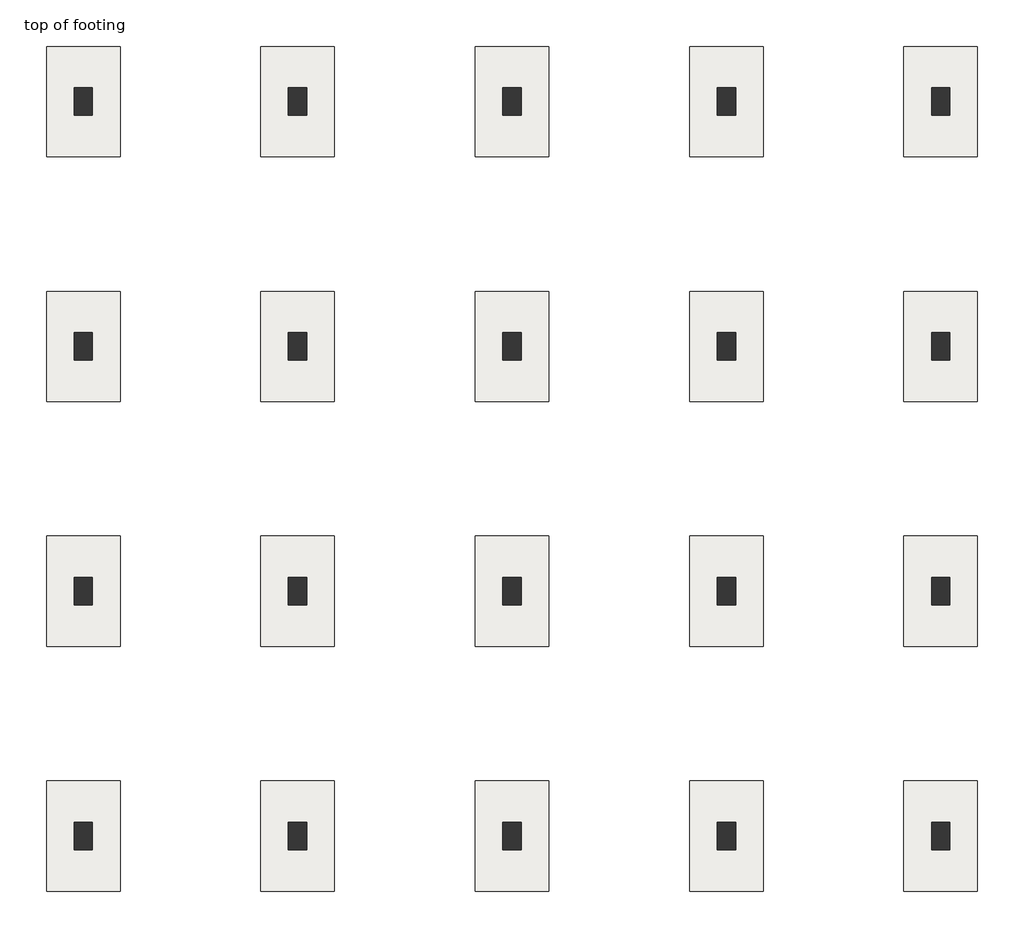
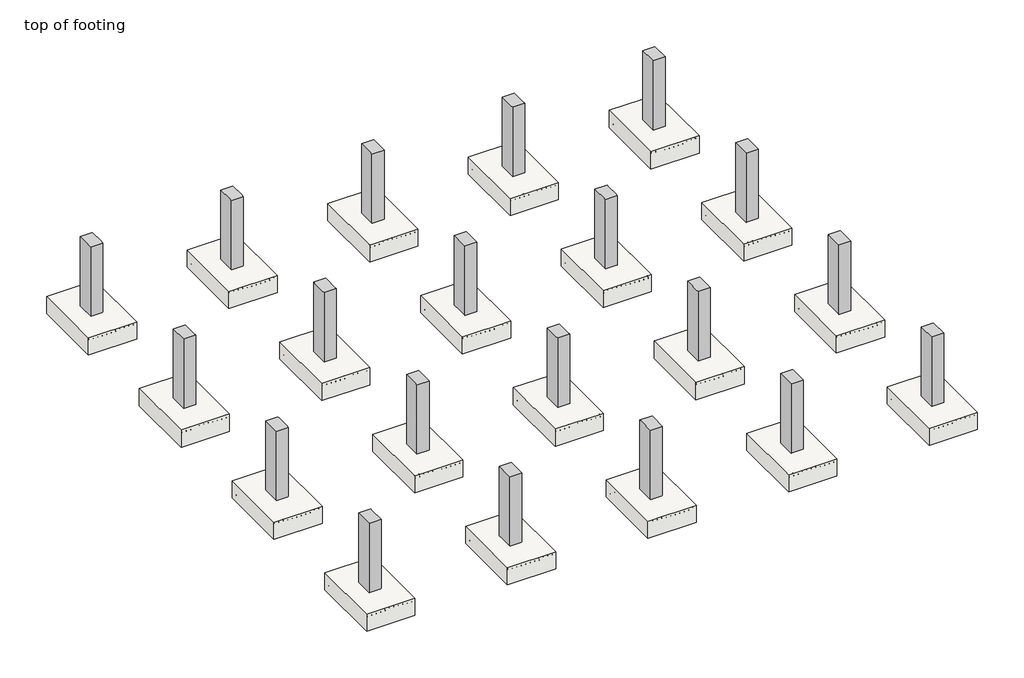
# One storey, part 1 of 8: 20 columns, 20 slabs.
"""IFC4 building model written with IfcOpenShell, lengths in millimetres."""

from ifc_helpers import new_model, si_unit, origin, place, context, project, spatial, faceted_brep, transform, mapped, element, save
from components import m_footing_rectangular_1800_x_1200_x_450mm_16ba7ea5

model = new_model("IFC4")

# Units and contexts
model_context = context("Model", 3, world=origin())
ifc_project = project(units=[si_unit("LENGTHUNIT", "METRE", prefix="MILLI")], contexts=[model_context])

# Site, building, storey
site = spatial("IfcSite", under=ifc_project)
building = spatial("IfcBuilding", under=site)
storey = spatial("IfcBuildingStorey", under=building, Name="top of footing", Elevation=-1828.8)

# Columns
placement = place(None, origin())
element("IfcColumn", 1, ObjectType="M_Concrete-Rectangular-Column : 300 x 450mm", at=placement, inside=storey, context=model_context, shape_type="Brep", body=[
    faceted_brep([(-11089.0800189, 17761.4575251, -1828.8), (-11089.0800189, 17311.4575251, -1828.8), (-11389.0800189, 17311.4575251, -1828.8), (-11389.0800189, 17761.4575251, -1828.8), (-11089.0800189, 17761.4575251, 0.0), (-11089.0800189, 17386.4575251, 0.0), (-11089.0800189, 17311.4575251, 0.0), (-11389.0800189, 17311.4575251, 0.0), (-11389.0800189, 17761.4575251, 0.0)], [[[0, 1, 2, 3]], [[4, 5, 6, 1, 0]], [[6, 7, 2, 1]], [[7, 8, 3, 2]], [[8, 4, 0, 3]], [[4, 8, 7, 6, 5]]]),
])
element("IfcColumn", 2, ObjectType="M_Concrete-Rectangular-Column : 300 x 450mm", at=placement, inside=storey, context=model_context, shape_type="Brep", body=[
    faceted_brep([(-11089.0800189, 13761.4575251, -1828.8), (-11089.0800189, 13311.4575251, -1828.8), (-11389.0800189, 13311.4575251, -1828.8), (-11389.0800189, 13761.4575251, -1828.8), (-11089.0800189, 13761.4575251, 0.0), (-11089.0800189, 13686.4575251, 0.0), (-11089.0800189, 13386.4575251, 0.0), (-11089.0800189, 13311.4575251, 0.0), (-11389.0800189, 13311.4575251, 0.0), (-11389.0800189, 13761.4575251, 0.0)], [[[0, 1, 2, 3]], [[4, 5, 6, 7, 1, 0]], [[7, 8, 2, 1]], [[8, 9, 3, 2]], [[9, 4, 0, 3]], [[4, 9, 8, 7, 6, 5]]]),
])
element("IfcColumn", 3, ObjectType="M_Concrete-Rectangular-Column : 300 x 450mm", at=placement, inside=storey, context=model_context, shape_type="Brep", body=[
    faceted_brep([(-11089.0800189, 9761.4575251, -1828.8), (-11089.0800189, 9311.4575251, -1828.8), (-11389.0800189, 9311.4575251, -1828.8), (-11389.0800189, 9761.4575251, -1828.8), (-11089.0800189, 9761.4575251, 0.0), (-11089.0800189, 9686.4575251, 0.0), (-11089.0800189, 9386.4575251, 0.0), (-11089.0800189, 9311.4575251, 0.0), (-11389.0800189, 9311.4575251, 0.0), (-11389.0800189, 9761.4575251, 0.0)], [[[0, 1, 2, 3]], [[4, 5, 6, 7, 1, 0]], [[7, 8, 2, 1]], [[8, 9, 3, 2]], [[9, 4, 0, 3]], [[4, 9, 8, 7, 6, 5]]]),
])
element("IfcColumn", 4, ObjectType="M_Concrete-Rectangular-Column : 300 x 450mm", at=placement, inside=storey, context=model_context, shape_type="Brep", body=[
    faceted_brep([(-11089.0800189, 5761.4575251, -1828.8), (-11089.0800189, 5311.4575251, -1828.8), (-11389.0800189, 5311.4575251, -1828.8), (-11389.0800189, 5761.4575251, -1828.8), (-11089.0800189, 5761.4575251, 0.0), (-11089.0800189, 5686.4575251, 0.0), (-11089.0800189, 5311.4575251, 0.0), (-11389.0800189, 5311.4575251, 0.0), (-11389.0800189, 5761.4575251, 0.0)], [[[0, 1, 2, 3]], [[4, 5, 6, 1, 0]], [[6, 7, 2, 1]], [[7, 8, 3, 2]], [[8, 4, 0, 3]], [[4, 8, 7, 6, 5]]]),
])
element("IfcColumn", 5, ObjectType="M_Concrete-Rectangular-Column : 300 x 450mm", at=placement, inside=storey, context=model_context, shape_type="Brep", body=[
    faceted_brep([(-7589.0800189, 17761.4575251, -1828.8), (-7589.0800189, 17311.4575251, -1828.8), (-7889.0800189, 17311.4575251, -1828.8), (-7889.0800189, 17761.4575251, -1828.8), (-7589.0800189, 17761.4575251, 0.0), (-7589.0800189, 17386.4575251, 0.0), (-7589.0800189, 17311.4575251, 0.0), (-7889.0800189, 17311.4575251, 0.0), (-7889.0800189, 17386.4575251, 0.0), (-7889.0800189, 17761.4575251, 0.0)], [[[0, 1, 2, 3]], [[4, 5, 6, 1, 0]], [[6, 7, 2, 1]], [[7, 8, 9, 3, 2]], [[9, 4, 0, 3]], [[4, 9, 8, 7, 6, 5]]]),
])
element("IfcColumn", 6, ObjectType="M_Concrete-Rectangular-Column : 300 x 450mm", at=placement, inside=storey, context=model_context, shape_type="Brep", body=[
    faceted_brep([(-7589.0800189, 13761.4575251, -1828.8), (-7589.0800189, 13311.4575251, -1828.8), (-7889.0800189, 13311.4575251, -1828.8), (-7889.0800189, 13761.4575251, -1828.8), (-7589.0800189, 13761.4575251, 0.0), (-7589.0800189, 13686.4575251, 0.0), (-7589.0800189, 13386.4575251, 0.0), (-7589.0800189, 13311.4575251, 0.0), (-7889.0800189, 13311.4575251, 0.0), (-7889.0800189, 13386.4575251, 0.0), (-7889.0800189, 13686.4575251, 0.0), (-7889.0800189, 13761.4575251, 0.0)], [[[0, 1, 2, 3]], [[4, 5, 6, 7, 1, 0]], [[7, 8, 2, 1]], [[8, 9, 10, 11, 3, 2]], [[11, 4, 0, 3]], [[4, 11, 10, 9, 8, 7, 6, 5]]]),
])
element("IfcColumn", 7, ObjectType="M_Concrete-Rectangular-Column : 300 x 450mm", at=placement, inside=storey, context=model_context, shape_type="Brep", body=[
    faceted_brep([(-7589.0800189, 9761.4575251, -1828.8), (-7589.0800189, 9311.4575251, -1828.8), (-7889.0800189, 9311.4575251, -1828.8), (-7889.0800189, 9761.4575251, -1828.8), (-7589.0800189, 9761.4575251, 0.0), (-7589.0800189, 9686.4575251, 0.0), (-7589.0800189, 9386.4575251, 0.0), (-7589.0800189, 9311.4575251, 0.0), (-7889.0800189, 9311.4575251, 0.0), (-7889.0800189, 9386.4575251, 0.0), (-7889.0800189, 9686.4575251, 0.0), (-7889.0800189, 9761.4575251, 0.0)], [[[0, 1, 2, 3]], [[4, 5, 6, 7, 1, 0]], [[7, 8, 2, 1]], [[8, 9, 10, 11, 3, 2]], [[11, 4, 0, 3]], [[4, 11, 10, 9, 8, 7, 6, 5]]]),
])
element("IfcColumn", 8, ObjectType="M_Concrete-Rectangular-Column : 300 x 450mm", at=placement, inside=storey, context=model_context, shape_type="Brep", body=[
    faceted_brep([(-7589.0800189, 5761.4575251, -1828.8), (-7589.0800189, 5311.4575251, -1828.8), (-7889.0800189, 5311.4575251, -1828.8), (-7889.0800189, 5761.4575251, -1828.8), (-7589.0800189, 5761.4575251, 0.0), (-7589.0800189, 5686.4575251, 0.0), (-7589.0800189, 5311.4575251, 0.0), (-7889.0800189, 5311.4575251, 0.0), (-7889.0800189, 5686.4575251, 0.0), (-7889.0800189, 5761.4575251, 0.0)], [[[0, 1, 2, 3]], [[4, 5, 6, 1, 0]], [[6, 7, 2, 1]], [[7, 8, 9, 3, 2]], [[9, 4, 0, 3]], [[4, 9, 8, 7, 6, 5]]]),
])
element("IfcColumn", 9, ObjectType="M_Concrete-Rectangular-Column : 300 x 450mm", at=placement, inside=storey, context=model_context, shape_type="Brep", body=[
    faceted_brep([(-4089.0800189, 17761.4575251, -1828.8), (-4089.0800189, 17311.4575251, -1828.8), (-4389.0800189, 17311.4575251, -1828.8), (-4389.0800189, 17761.4575251, -1828.8), (-4089.0800189, 17761.4575251, 0.0), (-4089.0800189, 17386.4575251, 0.0), (-4089.0800189, 17311.4575251, 0.0), (-4389.0800189, 17311.4575251, 0.0), (-4389.0800189, 17386.4575251, 0.0), (-4389.0800189, 17761.4575251, 0.0)], [[[0, 1, 2, 3]], [[4, 5, 6, 1, 0]], [[6, 7, 2, 1]], [[7, 8, 9, 3, 2]], [[9, 4, 0, 3]], [[4, 9, 8, 7, 6, 5]]]),
])
element("IfcColumn", 10, ObjectType="M_Concrete-Rectangular-Column : 300 x 450mm", at=placement, inside=storey, context=model_context, shape_type="Brep", body=[
    faceted_brep([(-4089.0800189, 13761.4575251, -1828.8), (-4089.0800189, 13311.4575251, -1828.8), (-4389.0800189, 13311.4575251, -1828.8), (-4389.0800189, 13761.4575251, -1828.8), (-4089.0800189, 13761.4575251, 0.0), (-4089.0800189, 13686.4575251, 0.0), (-4089.0800189, 13386.4575251, 0.0), (-4089.0800189, 13311.4575251, 0.0), (-4389.0800189, 13311.4575251, 0.0), (-4389.0800189, 13386.4575251, 0.0), (-4389.0800189, 13686.4575251, 0.0), (-4389.0800189, 13761.4575251, 0.0)], [[[0, 1, 2, 3]], [[4, 5, 6, 7, 1, 0]], [[7, 8, 2, 1]], [[8, 9, 10, 11, 3, 2]], [[11, 4, 0, 3]], [[4, 11, 10, 9, 8, 7, 6, 5]]]),
])
element("IfcColumn", 11, ObjectType="M_Concrete-Rectangular-Column : 300 x 450mm", at=placement, inside=storey, context=model_context, shape_type="Brep", body=[
    faceted_brep([(-4089.0800189, 9761.4575251, -1828.8), (-4089.0800189, 9311.4575251, -1828.8), (-4389.0800189, 9311.4575251, -1828.8), (-4389.0800189, 9761.4575251, -1828.8), (-4089.0800189, 9761.4575251, 0.0), (-4089.0800189, 9686.4575251, 0.0), (-4089.0800189, 9386.4575251, 0.0), (-4089.0800189, 9311.4575251, 0.0), (-4389.0800189, 9311.4575251, 0.0), (-4389.0800189, 9386.4575251, 0.0), (-4389.0800189, 9686.4575251, 0.0), (-4389.0800189, 9761.4575251, 0.0)], [[[0, 1, 2, 3]], [[4, 5, 6, 7, 1, 0]], [[7, 8, 2, 1]], [[8, 9, 10, 11, 3, 2]], [[11, 4, 0, 3]], [[4, 11, 10, 9, 8, 7, 6, 5]]]),
])
element("IfcColumn", 12, ObjectType="M_Concrete-Rectangular-Column : 300 x 450mm", at=placement, inside=storey, context=model_context, shape_type="Brep", body=[
    faceted_brep([(-4089.0800189, 5761.4575251, -1828.8), (-4089.0800189, 5311.4575251, -1828.8), (-4389.0800189, 5311.4575251, -1828.8), (-4389.0800189, 5761.4575251, -1828.8), (-4089.0800189, 5761.4575251, 0.0), (-4089.0800189, 5686.4575251, 0.0), (-4089.0800189, 5311.4575251, 0.0), (-4389.0800189, 5311.4575251, 0.0), (-4389.0800189, 5686.4575251, 0.0), (-4389.0800189, 5761.4575251, 0.0)], [[[0, 1, 2, 3]], [[4, 5, 6, 1, 0]], [[6, 7, 2, 1]], [[7, 8, 9, 3, 2]], [[9, 4, 0, 3]], [[4, 9, 8, 7, 6, 5]]]),
])
element("IfcColumn", 13, ObjectType="M_Concrete-Rectangular-Column : 300 x 450mm", at=placement, inside=storey, context=model_context, shape_type="Brep", body=[
    faceted_brep([(-589.0800189, 17761.4575251, -1828.8), (-589.0800189, 17311.4575251, -1828.8), (-889.0800189, 17311.4575251, -1828.8), (-889.0800189, 17761.4575251, -1828.8), (-589.0800189, 17761.4575251, 0.0), (-589.0800189, 17386.4575251, 0.0), (-589.0800189, 17311.4575251, 0.0), (-889.0800189, 17311.4575251, 0.0), (-889.0800189, 17386.4575251, 0.0), (-889.0800189, 17761.4575251, 0.0)], [[[0, 1, 2, 3]], [[4, 5, 6, 1, 0]], [[6, 7, 2, 1]], [[7, 8, 9, 3, 2]], [[9, 4, 0, 3]], [[4, 9, 8, 7, 6, 5]]]),
])
element("IfcColumn", 14, ObjectType="M_Concrete-Rectangular-Column : 300 x 450mm", at=placement, inside=storey, context=model_context, shape_type="Brep", body=[
    faceted_brep([(-589.0800189, 13761.4575251, -1828.8), (-589.0800189, 13311.4575251, -1828.8), (-889.0800189, 13311.4575251, -1828.8), (-889.0800189, 13761.4575251, -1828.8), (-589.0800189, 13761.4575251, 0.0), (-589.0800189, 13686.4575251, 0.0), (-589.0800189, 13386.4575251, 0.0), (-589.0800189, 13311.4575251, 0.0), (-889.0800189, 13311.4575251, 0.0), (-889.0800189, 13386.4575251, 0.0), (-889.0800189, 13686.4575251, 0.0), (-889.0800189, 13761.4575251, 0.0)], [[[0, 1, 2, 3]], [[4, 5, 6, 7, 1, 0]], [[7, 8, 2, 1]], [[8, 9, 10, 11, 3, 2]], [[11, 4, 0, 3]], [[4, 11, 10, 9, 8, 7, 6, 5]]]),
])
element("IfcColumn", 15, ObjectType="M_Concrete-Rectangular-Column : 300 x 450mm", at=placement, inside=storey, context=model_context, shape_type="Brep", body=[
    faceted_brep([(-589.0800189, 9761.4575251, -1828.8), (-589.0800189, 9311.4575251, -1828.8), (-889.0800189, 9311.4575251, -1828.8), (-889.0800189, 9761.4575251, -1828.8), (-589.0800189, 9761.4575251, 0.0), (-589.0800189, 9686.4575251, 0.0), (-589.0800189, 9386.4575251, 0.0), (-589.0800189, 9311.4575251, 0.0), (-889.0800189, 9311.4575251, 0.0), (-889.0800189, 9386.4575251, 0.0), (-889.0800189, 9686.4575251, 0.0), (-889.0800189, 9761.4575251, 0.0)], [[[0, 1, 2, 3]], [[4, 5, 6, 7, 1, 0]], [[7, 8, 2, 1]], [[8, 9, 10, 11, 3, 2]], [[11, 4, 0, 3]], [[4, 11, 10, 9, 8, 7, 6, 5]]]),
])
element("IfcColumn", 16, ObjectType="M_Concrete-Rectangular-Column : 300 x 450mm", at=placement, inside=storey, context=model_context, shape_type="Brep", body=[
    faceted_brep([(-589.0800189, 5761.4575251, -1828.8), (-589.0800189, 5311.4575251, -1828.8), (-889.0800189, 5311.4575251, -1828.8), (-889.0800189, 5761.4575251, -1828.8), (-589.0800189, 5761.4575251, 0.0), (-589.0800189, 5686.4575251, 0.0), (-589.0800189, 5311.4575251, 0.0), (-889.0800189, 5311.4575251, 0.0), (-889.0800189, 5686.4575251, 0.0), (-889.0800189, 5761.4575251, 0.0)], [[[0, 1, 2, 3]], [[4, 5, 6, 1, 0]], [[6, 7, 2, 1]], [[7, 8, 9, 3, 2]], [[9, 4, 0, 3]], [[4, 9, 8, 7, 6, 5]]]),
])
element("IfcColumn", 17, ObjectType="M_Concrete-Rectangular-Column : 300 x 450mm", at=placement, inside=storey, context=model_context, shape_type="Brep", body=[
    faceted_brep([(2910.9199811, 17761.4575251, -1828.8), (2910.9199811, 17311.4575251, -1828.8), (2610.9199811, 17311.4575251, -1828.8), (2610.9199811, 17761.4575251, -1828.8), (2910.9199811, 17761.4575251, 0.0), (2910.9199811, 17311.4575251, 0.0), (2610.9199811, 17311.4575251, 0.0), (2610.9199811, 17386.4575251, 0.0), (2610.9199811, 17761.4575251, 0.0)], [[[0, 1, 2, 3]], [[4, 5, 1, 0]], [[5, 6, 2, 1]], [[6, 7, 8, 3, 2]], [[8, 4, 0, 3]], [[4, 8, 7, 6, 5]]]),
])
element("IfcColumn", 18, ObjectType="M_Concrete-Rectangular-Column : 300 x 450mm", at=placement, inside=storey, context=model_context, shape_type="Brep", body=[
    faceted_brep([(2910.9199811, 13761.4575251, -1828.8), (2910.9199811, 13311.4575251, -1828.8), (2610.9199811, 13311.4575251, -1828.8), (2610.9199811, 13761.4575251, -1828.8), (2910.9199811, 13761.4575251, 0.0), (2910.9199811, 13311.4575251, 0.0), (2610.9199811, 13311.4575251, 0.0), (2610.9199811, 13386.4575251, 0.0), (2610.9199811, 13686.4575251, 0.0), (2610.9199811, 13761.4575251, 0.0)], [[[0, 1, 2, 3]], [[4, 5, 1, 0]], [[5, 6, 2, 1]], [[6, 7, 8, 9, 3, 2]], [[9, 4, 0, 3]], [[4, 9, 8, 7, 6, 5]]]),
])
element("IfcColumn", 19, ObjectType="M_Concrete-Rectangular-Column : 300 x 450mm", at=placement, inside=storey, context=model_context, shape_type="Brep", body=[
    faceted_brep([(2910.9199811, 9761.4575251, -1828.8), (2910.9199811, 9311.4575251, -1828.8), (2610.9199811, 9311.4575251, -1828.8), (2610.9199811, 9761.4575251, -1828.8), (2910.9199811, 9761.4575251, 0.0), (2910.9199811, 9311.4575251, 0.0), (2610.9199811, 9311.4575251, 0.0), (2610.9199811, 9386.4575251, 0.0), (2610.9199811, 9686.4575251, 0.0), (2610.9199811, 9761.4575251, 0.0)], [[[0, 1, 2, 3]], [[4, 5, 1, 0]], [[5, 6, 2, 1]], [[6, 7, 8, 9, 3, 2]], [[9, 4, 0, 3]], [[4, 9, 8, 7, 6, 5]]]),
])
element("IfcColumn", 20, ObjectType="M_Concrete-Rectangular-Column : 300 x 450mm", at=placement, inside=storey, context=model_context, shape_type="Brep", body=[
    faceted_brep([(2910.9199811, 5761.4575251, -1828.8), (2910.9199811, 5311.4575251, -1828.8), (2610.9199811, 5311.4575251, -1828.8), (2610.9199811, 5761.4575251, -1828.8), (2910.9199811, 5761.4575251, 0.0), (2910.9199811, 5311.4575251, 0.0), (2610.9199811, 5311.4575251, 0.0), (2610.9199811, 5686.4575251, 0.0), (2610.9199811, 5761.4575251, 0.0)], [[[0, 1, 2, 3]], [[4, 5, 1, 0]], [[5, 6, 2, 1]], [[6, 7, 8, 3, 2]], [[8, 4, 0, 3]], [[4, 8, 7, 6, 5]]]),
])

# Slabs
m_footing_rectangular_1800_x_1200_x_450mm_shape = m_footing_rectangular_1800_x_1200_x_450mm_16ba7ea5(model_context)
element("IfcSlab", 21, ObjectType="M_Footing-Rectangular : 1800 x 1200 x 450mm", at=placement, inside=storey, context=model_context, shape_type="MappedRepresentation", body=[
    mapped(m_footing_rectangular_1800_x_1200_x_450mm_shape, transform((-11239.0800189, 17536.4575251, -1828.8), x_axis=(1.0, 0.0, 0.0), y_axis=(0.0, 1.0, 0.0), z_axis=(0.0, 0.0, 1.0))),
])
element("IfcSlab", 22, ObjectType="M_Footing-Rectangular : 1800 x 1200 x 450mm", at=placement, inside=storey, context=model_context, shape_type="MappedRepresentation", body=[
    mapped(m_footing_rectangular_1800_x_1200_x_450mm_shape, transform((-11239.0800189, 13536.4575251, -1828.8), x_axis=(1.0, 0.0, 0.0), y_axis=(0.0, 1.0, 0.0), z_axis=(0.0, 0.0, 1.0))),
])
element("IfcSlab", 23, ObjectType="M_Footing-Rectangular : 1800 x 1200 x 450mm", at=placement, inside=storey, context=model_context, shape_type="MappedRepresentation", body=[
    mapped(m_footing_rectangular_1800_x_1200_x_450mm_shape, transform((-11239.0800189, 9536.4575251, -1828.8), x_axis=(1.0, 0.0, 0.0), y_axis=(0.0, 1.0, 0.0), z_axis=(0.0, 0.0, 1.0))),
])
element("IfcSlab", 24, ObjectType="M_Footing-Rectangular : 1800 x 1200 x 450mm", at=placement, inside=storey, context=model_context, shape_type="MappedRepresentation", body=[
    mapped(m_footing_rectangular_1800_x_1200_x_450mm_shape, transform((-11239.0800189, 5536.4575251, -1828.8), x_axis=(1.0, 0.0, 0.0), y_axis=(0.0, 1.0, 0.0), z_axis=(0.0, 0.0, 1.0))),
])
element("IfcSlab", 25, ObjectType="M_Footing-Rectangular : 1800 x 1200 x 450mm", at=placement, inside=storey, context=model_context, shape_type="MappedRepresentation", body=[
    mapped(m_footing_rectangular_1800_x_1200_x_450mm_shape, transform((-7739.0800189, 17536.4575251, -1828.8), x_axis=(1.0, 0.0, 0.0), y_axis=(0.0, 1.0, 0.0), z_axis=(0.0, 0.0, 1.0))),
])
element("IfcSlab", 26, ObjectType="M_Footing-Rectangular : 1800 x 1200 x 450mm", at=placement, inside=storey, context=model_context, shape_type="MappedRepresentation", body=[
    mapped(m_footing_rectangular_1800_x_1200_x_450mm_shape, transform((-7739.0800189, 13536.4575251, -1828.8), x_axis=(1.0, 0.0, 0.0), y_axis=(0.0, 1.0, 0.0), z_axis=(0.0, 0.0, 1.0))),
])
element("IfcSlab", 27, ObjectType="M_Footing-Rectangular : 1800 x 1200 x 450mm", at=placement, inside=storey, context=model_context, shape_type="MappedRepresentation", body=[
    mapped(m_footing_rectangular_1800_x_1200_x_450mm_shape, transform((-7739.0800189, 9536.4575251, -1828.8), x_axis=(1.0, 0.0, 0.0), y_axis=(0.0, 1.0, 0.0), z_axis=(0.0, 0.0, 1.0))),
])
element("IfcSlab", 28, ObjectType="M_Footing-Rectangular : 1800 x 1200 x 450mm", at=placement, inside=storey, context=model_context, shape_type="MappedRepresentation", body=[
    mapped(m_footing_rectangular_1800_x_1200_x_450mm_shape, transform((-7739.0800189, 5536.4575251, -1828.8), x_axis=(1.0, 0.0, 0.0), y_axis=(0.0, 1.0, 0.0), z_axis=(0.0, 0.0, 1.0))),
])
element("IfcSlab", 29, ObjectType="M_Footing-Rectangular : 1800 x 1200 x 450mm", at=placement, inside=storey, context=model_context, shape_type="MappedRepresentation", body=[
    mapped(m_footing_rectangular_1800_x_1200_x_450mm_shape, transform((-4239.0800189, 17536.4575251, -1828.8), x_axis=(1.0, 0.0, 0.0), y_axis=(0.0, 1.0, 0.0), z_axis=(0.0, 0.0, 1.0))),
])
element("IfcSlab", 30, ObjectType="M_Footing-Rectangular : 1800 x 1200 x 450mm", at=placement, inside=storey, context=model_context, shape_type="MappedRepresentation", body=[
    mapped(m_footing_rectangular_1800_x_1200_x_450mm_shape, transform((-4239.0800189, 13536.4575251, -1828.8), x_axis=(1.0, 0.0, 0.0), y_axis=(0.0, 1.0, 0.0), z_axis=(0.0, 0.0, 1.0))),
])
element("IfcSlab", 31, ObjectType="M_Footing-Rectangular : 1800 x 1200 x 450mm", at=placement, inside=storey, context=model_context, shape_type="MappedRepresentation", body=[
    mapped(m_footing_rectangular_1800_x_1200_x_450mm_shape, transform((-4239.0800189, 9536.4575251, -1828.8), x_axis=(1.0, 0.0, 0.0), y_axis=(0.0, 1.0, 0.0), z_axis=(0.0, 0.0, 1.0))),
])
element("IfcSlab", 32, ObjectType="M_Footing-Rectangular : 1800 x 1200 x 450mm", at=placement, inside=storey, context=model_context, shape_type="MappedRepresentation", body=[
    mapped(m_footing_rectangular_1800_x_1200_x_450mm_shape, transform((-4239.0800189, 5536.4575251, -1828.8), x_axis=(1.0, 0.0, 0.0), y_axis=(0.0, 1.0, 0.0), z_axis=(0.0, 0.0, 1.0))),
])
element("IfcSlab", 33, ObjectType="M_Footing-Rectangular : 1800 x 1200 x 450mm", at=placement, inside=storey, context=model_context, shape_type="MappedRepresentation", body=[
    mapped(m_footing_rectangular_1800_x_1200_x_450mm_shape, transform((-739.0800189, 17536.4575251, -1828.8), x_axis=(1.0, 0.0, 0.0), y_axis=(0.0, 1.0, 0.0), z_axis=(0.0, 0.0, 1.0))),
])
element("IfcSlab", 34, ObjectType="M_Footing-Rectangular : 1800 x 1200 x 450mm", at=placement, inside=storey, context=model_context, shape_type="MappedRepresentation", body=[
    mapped(m_footing_rectangular_1800_x_1200_x_450mm_shape, transform((-739.0800189, 13536.4575251, -1828.8), x_axis=(1.0, 0.0, 0.0), y_axis=(0.0, 1.0, 0.0), z_axis=(0.0, 0.0, 1.0))),
])
element("IfcSlab", 35, ObjectType="M_Footing-Rectangular : 1800 x 1200 x 450mm", at=placement, inside=storey, context=model_context, shape_type="MappedRepresentation", body=[
    mapped(m_footing_rectangular_1800_x_1200_x_450mm_shape, transform((-739.0800189, 9536.4575251, -1828.8), x_axis=(1.0, 0.0, 0.0), y_axis=(0.0, 1.0, 0.0), z_axis=(0.0, 0.0, 1.0))),
])
element("IfcSlab", 36, ObjectType="M_Footing-Rectangular : 1800 x 1200 x 450mm", at=placement, inside=storey, context=model_context, shape_type="MappedRepresentation", body=[
    mapped(m_footing_rectangular_1800_x_1200_x_450mm_shape, transform((-739.0800189, 5536.4575251, -1828.8), x_axis=(1.0, 0.0, 0.0), y_axis=(0.0, 1.0, 0.0), z_axis=(0.0, 0.0, 1.0))),
])
element("IfcSlab", 37, ObjectType="M_Footing-Rectangular : 1800 x 1200 x 450mm", at=placement, inside=storey, context=model_context, shape_type="MappedRepresentation", body=[
    mapped(m_footing_rectangular_1800_x_1200_x_450mm_shape, transform((2760.9199811, 17536.4575251, -1828.8), x_axis=(1.0, 0.0, 0.0), y_axis=(0.0, 1.0, 0.0), z_axis=(0.0, 0.0, 1.0))),
])
element("IfcSlab", 38, ObjectType="M_Footing-Rectangular : 1800 x 1200 x 450mm", at=placement, inside=storey, context=model_context, shape_type="MappedRepresentation", body=[
    mapped(m_footing_rectangular_1800_x_1200_x_450mm_shape, transform((2760.9199811, 13536.4575251, -1828.8), x_axis=(1.0, 0.0, 0.0), y_axis=(0.0, 1.0, 0.0), z_axis=(0.0, 0.0, 1.0))),
])
element("IfcSlab", 39, ObjectType="M_Footing-Rectangular : 1800 x 1200 x 450mm", at=placement, inside=storey, context=model_context, shape_type="MappedRepresentation", body=[
    mapped(m_footing_rectangular_1800_x_1200_x_450mm_shape, transform((2760.9199811, 9536.4575251, -1828.8), x_axis=(1.0, 0.0, 0.0), y_axis=(0.0, 1.0, 0.0), z_axis=(0.0, 0.0, 1.0))),
])
element("IfcSlab", 40, ObjectType="M_Footing-Rectangular : 1800 x 1200 x 450mm", at=placement, inside=storey, context=model_context, shape_type="MappedRepresentation", body=[
    mapped(m_footing_rectangular_1800_x_1200_x_450mm_shape, transform((2760.9199811, 5536.4575251, -1828.8), x_axis=(1.0, 0.0, 0.0), y_axis=(0.0, 1.0, 0.0), z_axis=(0.0, 0.0, 1.0))),
])

save(model, "model.ifc")

# Revit data of these elements
# Grids (mm)
#   "1": line (-11239.08, 21848.332) -> (-11239.08, -15769.142)
#   "2": line (-7739.08, 21848.332) -> (-7739.08, -15769.142)
#   "3": line (-4239.08, 21848.332) -> (-4239.08, -15769.142)
#   "4": line (-739.08, 21848.332) -> (-739.08, -15769.142)
#   "5": line (2760.92, 21848.332) -> (2760.92, -15769.142)
#   "A": line (7472.497, 17536.458) -> (-13539.968, 17536.458)
#   "B": line (7472.497, 13536.458) -> (-13539.968, 13536.458)
#   "C": line (7472.497, 9536.458) -> (-13539.968, 9536.458)
#   "D": line (7472.497, 5536.458) -> (-13539.968, 5536.458)
# Type "M_Concrete-Rectangular-Column : 300 x 450mm"
#   b = 0' - 11.81102"
#   h = 1' - 5.71654"
#   Structural Material [instance default] = Concrete, Cast-in-Place gray
# Type "M_Footing-Rectangular : 1800 x 1200 x 450mm"
#   Width = 3' - 11.24409"
#   Length = 5' - 10.86614"
#   Foundation Thickness = 1' - 5.71654"
#   Structural Material [instance default] = Concrete, Cast-in-Place gray
#   Assembly Code = ""
# Elements 1, 2, 3, 4, 5, 6, 7, 8, 9, 10, 11, 12, 13, 14, 15, 16, 17, 18, 19, 20 (IfcColumn, "M_Concrete-Rectangular-Column : 300 x 450mm")
#   Structural Material = Concrete, Cast-in-Place gray
#   Phase Created = New Construction
#   Materials on its faces: "Concrete, Cast-in-Place gray"
# Elements 21, 22, 23, 24, 25, 26, 27, 28, 29, 30, 31, 32, 33, 34, 35, 36, 37, 38, 39, 40 (IfcSlab, "M_Footing-Rectangular : 1800 x 1200 x 450mm")
#   Structural Material = Concrete, Cast-in-Place gray
#   Phase Created = New Construction
#   Materials on its faces: "Concrete, Cast-in-Place gray"
# Materials
#   "Concrete, Cast-in-Place gray": class "Concrete", colour RGB 192 192 192, transparency 0, Description = "Cast-in-place concrete", Cost = 0
